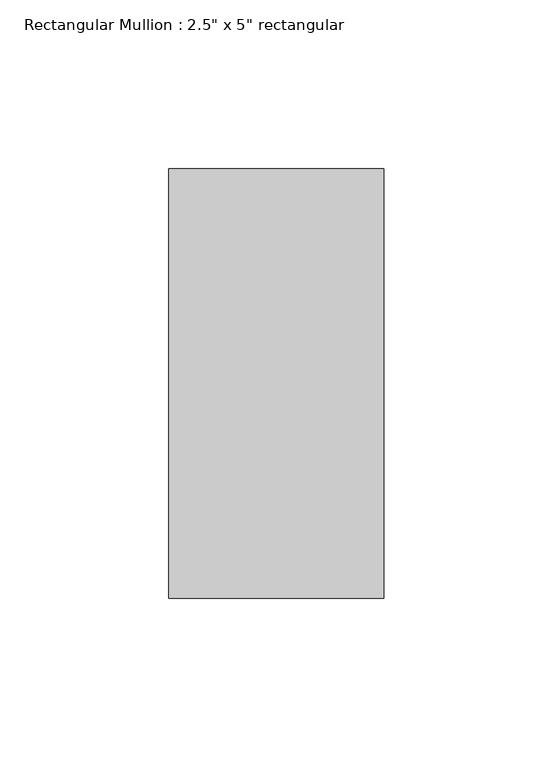
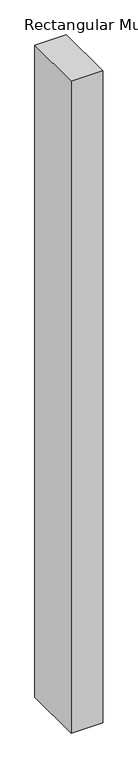
"""IFC4 building model written with IfcOpenShell, lengths in millimetres: member geometry."""

from ifc_helpers import new_model, si_unit, frame, origin, place, context, project, spatial, polyline, outline, extrude, source, transform, mapped, element, save


def member_a36b500a(model_context):
    return source(origin(), model_context, "Body", "SweptSolid", [
        extrude(outline(polyline([(0.0, 63.5), (0.0, -63.5), (-63.5, -63.5), (-63.5, 63.5), (0.0, 63.5)])), frame((0.0, 0.0, -1390.65), z_axis=(0.0, 0.0, 1.0), x_axis=(1.0, 0.0, 0.0)), (0.0, 0.0, 1.0), 1390.65),
    ])


if __name__ == "__main__":
    model = new_model("IFC4")
    model_context = context("Model", 3, world=origin())
    ifc_project = project(units=[si_unit("LENGTHUNIT", "METRE", prefix="MILLI")], contexts=[model_context])
    site = spatial("IfcSite", under=ifc_project)
    building = spatial("IfcBuilding", under=site)
    placement = place(None, origin())
    member_shape = member_a36b500a(model_context)
    element("IfcMember", 1, ObjectType="Rectangular Mullion : 2.5\" x 5\" rectangular", at=placement, inside=building, context=model_context, shape_type="MappedRepresentation", body=[
        mapped(member_shape, transform((0.0, 0.0, 0.0), x_axis=(1.0, 0.0, 0.0), y_axis=(0.0, 1.0, 0.0), z_axis=(0.0, 0.0, 1.0))),
    ])
    save(model, "model.ifc")

# Revit data of these elements
# Type "Rectangular Mullion : 2.5\" x 5\" rectangular"
#   built-in parameter 1007304 = 0.416667 (stored number, unit not read)
#   built-in parameter 1007301 = 0.104167 (stored number, unit not read)
#   built-in parameter 1007300 = 0.104167 (stored number, unit not read)
# Element 1 (IfcMember, "Rectangular Mullion : 2.5\" x 5\" rectangular")
#   Materials on its faces: "Aluminum"
# Materials
#   "Aluminum": class "Metal", colour RGB 247 247 247, transparency 0, Description = "Aluminum 6061", Cost = 0
